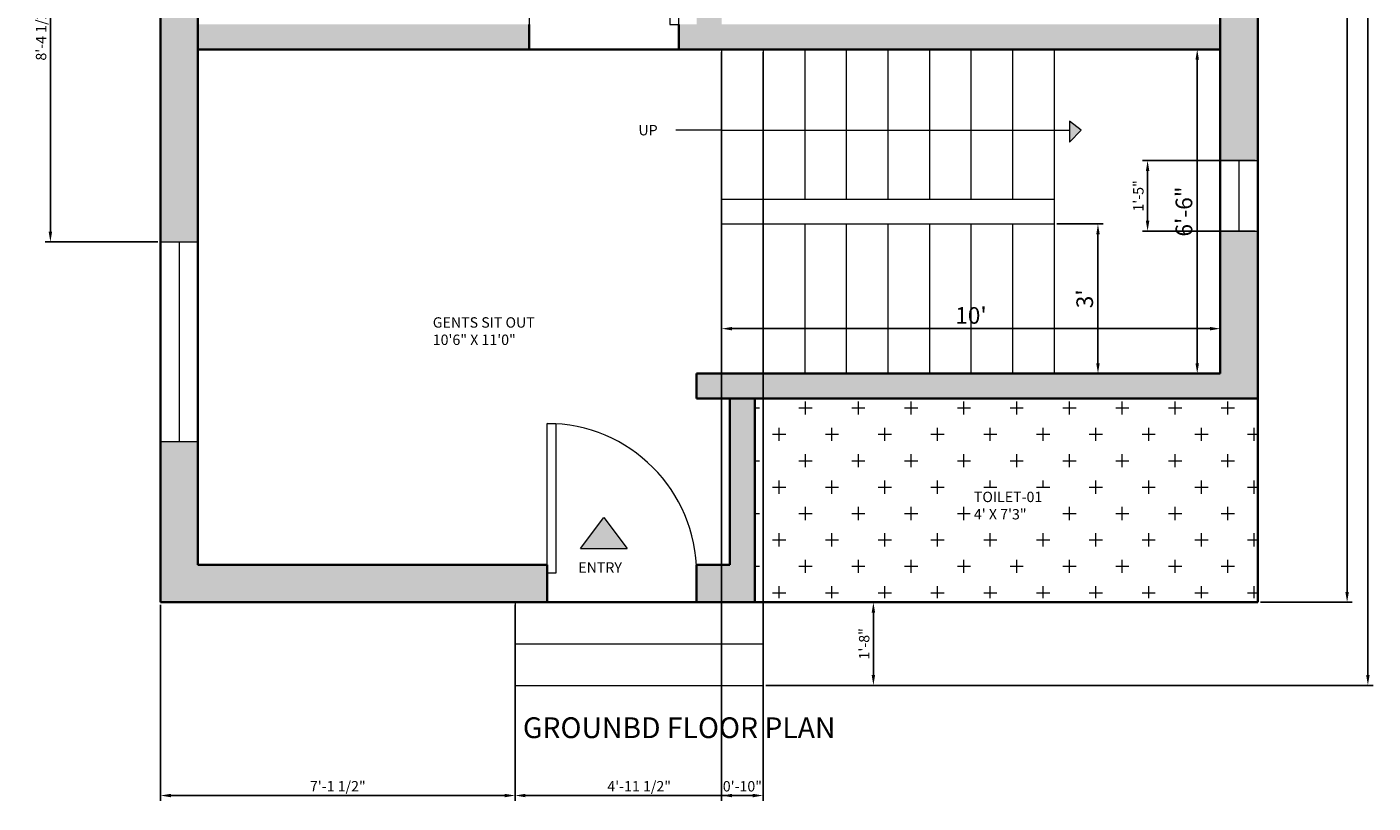
# Model space of a CAD drawing. Units: inches. Extents: x 5395 to 6469, y -203 to 448.
# Tile 6 of 7: x 6145 to 6469, y -203 to -16. Entities that reach past the tile are written whole.
import ezdxf

# ---------------------------------------------------------------- set-up
doc = ezdxf.new("R2010")
doc.units = ezdxf.units.IN
for name, color, linetype, lineweight in [('A-ANNO-DIMS', 2, 'Continuous', 18), ('A-ANNO-SYMB', 3, 'Continuous', 18), ('A-ANNO-TEXT', 6, 'Continuous', 18), ('A-AREA-IDEN', 6, 'Continuous', 18), ('A-FLOR-PATT', 3, 'Continuous', 13), ('A-FLOR-STRS', 3, 'Continuous', 18), ('A-GLAZ', 4, 'Continuous', 18), ('A-WALL', 7, 'Continuous', 35), ('A-WALL-PATT', 11, 'Continuous', 9), ('door', 240, 'Continuous', 18)]:
    doc.layers.add(name, color=color, linetype=linetype, lineweight=lineweight)
doc.styles.get("Standard").update_dxf_attribs({"font": 'arial.ttf'})
doc.dimstyles.new('ISO-25', dxfattribs={"dimtxt": 2.5, "dimasz": 2.5, "dimexe": 1.25, "dimexo": 0.625, "dimtad": 1, "dimdec": 1, "dimlunit": 3, "dimtxsty": 'Standard', "dimcen": 2.5, "dimadec": 0, "dimazin": 0, "dimtfac": 1, "dimtdec": 1, "dimtmove": 0, "dimatfit": 3, "dimfxl": 1, "dimarcsym": 0})

# ---------------------------------------------------------------- blocks, each defined once
blk = doc.blocks.new('*D23')
at = {"layer": 'A-ANNO-DIMS', "color": 0, "lineweight": -2, "transparency": 16777216}
for p, q in [((6421.36, -21.69), (6428.02, -21.69)), ((6426.77, -24.19), (6426.77, -97.19)), ((6427.4, -99.69), (6428.02, -99.69))]:
    blk.add_line(p, q, dxfattribs=at)
at = {"layer": 'A-ANNO-DIMS', "color": 0, "transparency": 16777216}
for points in [[(6426.35, -24.19), (6427.19, -24.19), (6426.77, -21.69)], [(6426.35, -97.19), (6427.19, -97.19), (6426.77, -99.69)]]:
    blk.add_solid(points, dxfattribs=at)
at = {"layer": 'Defpoints', "color": 0, "transparency": 16777216}
for p in [(6420.73, -21.69), (6426.77, -99.69), (6426.77, -99.69)]:
    blk.add_point(p, dxfattribs=at)
at = {"layer": 'A-ANNO-DIMS', "color": 0, "transparency": 16777216, "insert": (6424.1, -60.69), "char_height": 4, "attachment_point": 5, "rotation": 90}
blk.add_mtext('6\'-6"', dxfattribs=at)
blk = doc.blocks.new('*D24')
at = {"layer": 'A-ANNO-DIMS', "color": 0, "lineweight": -2, "transparency": 16777216}
for p, q in [((6392.96, -63.69), (6404.14, -63.69)), ((6402.89, -66.19), (6402.89, -97.19)), ((6392.96, -99.69), (6404.14, -99.69))]:
    blk.add_line(p, q, dxfattribs=at)
at = {"layer": 'A-ANNO-DIMS', "color": 0, "transparency": 16777216}
for points in [[(6402.48, -66.19), (6403.31, -66.19), (6402.89, -63.69)], [(6402.48, -97.19), (6403.31, -97.19), (6402.89, -99.69)]]:
    blk.add_solid(points, dxfattribs=at)
at = {"layer": 'Defpoints', "color": 0, "transparency": 16777216}
for p in [(6392.33, -63.69), (6392.33, -99.69), (6402.89, -99.69)]:
    blk.add_point(p, dxfattribs=at)
at = {"layer": 'A-ANNO-DIMS', "color": 0, "transparency": 16777216, "insert": (6400.22, -81.69), "char_height": 4, "attachment_point": 5, "rotation": 90}
blk.add_mtext("3'", dxfattribs=at)
blk = doc.blocks.new('*D25')
at = {"layer": 'A-ANNO-DIMS', "color": 0, "lineweight": -2, "transparency": 16777216}
for p, q in [((6312.33, -41.76), (6312.33, -90.12)), ((6432.33, -41.76), (6432.33, -90.12)), ((6314.83, -88.87), (6429.83, -88.87))]:
    blk.add_line(p, q, dxfattribs=at)
at = {"layer": 'A-ANNO-DIMS', "color": 0, "transparency": 16777216}
for points in [[(6314.83, -88.46), (6314.83, -89.29), (6312.33, -88.87)], [(6429.83, -88.46), (6429.83, -89.29), (6432.33, -88.87)]]:
    blk.add_solid(points, dxfattribs=at)
at = {"layer": 'Defpoints', "color": 0, "transparency": 16777216}
for p in [(6312.33, -41.13), (6432.33, -41.13), (6432.33, -88.87)]:
    blk.add_point(p, dxfattribs=at)
at = {"layer": 'A-ANNO-DIMS', "color": 0, "transparency": 16777216, "insert": (6372.33, -86.21), "char_height": 4, "attachment_point": 5}
blk.add_mtext("10'", dxfattribs=at)
blk = doc.blocks.new('*U3')
for p, q in [((-30, 0), (-30, -5)), ((0, 0), (0, -5))]:
    blk.add_line(p, q)
blk.add_lwpolyline([(0, 0), (0, 30), (-1.75, 30), (-1.75, 0)], close=True)
blk.add_arc((0, 0), 30, 90, 180)
blk = doc.blocks.new('*U2')
for p, q in [((0, 0), (0, -5)), ((30, 0), (30, -5))]:
    blk.add_line(p, q)
blk.add_lwpolyline([(0, 0), (0, 30), (1.75, 30), (1.75, 0)], close=True)
blk.add_arc((0, 0), 30, 0, 90)
blk = doc.blocks.new('*D28')
at = {"layer": 'A-ANNO-DIMS', "color": 0, "lineweight": -2, "transparency": 16777216}
for p, q in [((6441.96, 325.31), (6464.09, 325.31)), ((6462.84, 322.81), (6462.84, -152.19)), ((6441.96, -154.69), (6464.09, -154.69))]:
    blk.add_line(p, q, dxfattribs=at)
at = {"layer": 'A-ANNO-DIMS', "color": 0, "transparency": 16777216}
for points in [[(6462.42, 322.81), (6463.25, 322.81), (6462.84, 325.31)], [(6462.42, -152.19), (6463.25, -152.19), (6462.84, -154.69)]]:
    blk.add_solid(points, dxfattribs=at)
at = {"layer": 'Defpoints', "color": 0, "transparency": 16777216}
for p in [(6441.33, 325.31), (6441.33, -154.69), (6462.84, -154.69)]:
    blk.add_point(p, dxfattribs=at)
at = {"layer": 'A-ANNO-DIMS', "color": 0, "transparency": 16777216, "insert": (6460.17, 85.31), "char_height": 4, "attachment_point": 5, "rotation": 90}
blk.add_mtext("40'", dxfattribs=at)
blk = doc.blocks.new('WINDOW-48IN')
for p, q in [((0, 0), (0, 9)), ((48, 0), (48, 9)), ((0, 4.5), (48, 4.5))]:
    blk.add_line(p, q)
blk = doc.blocks.new('*D77')
at = {"layer": 'A-ANNO-DIMS', "color": 0, "lineweight": -2, "transparency": 16777216}
for p, q in [((6176.71, 32.67), (6149.58, 32.67)), ((6150.83, 30.17), (6150.83, -65.51)), ((6176.71, -68.01), (6149.58, -68.01))]:
    blk.add_line(p, q, dxfattribs=at)
at = {"layer": 'A-ANNO-DIMS', "color": 0, "transparency": 16777216}
for points in [[(6150.42, 30.17), (6151.25, 30.17), (6150.83, 32.67)], [(6150.42, -65.51), (6151.25, -65.51), (6150.83, -68.01)]]:
    blk.add_solid(points, dxfattribs=at)
at = {"layer": 'Defpoints', "color": 0, "transparency": 16777216}
for p in [(6177.33, 32.67), (6150.83, -68.01), (6177.33, -68.01)]:
    blk.add_point(p, dxfattribs=at)
at = {"layer": 'A-ANNO-DIMS', "color": 0, "transparency": 16777216, "insert": (6148.92, -17.67), "char_height": 2.5, "attachment_point": 5, "rotation": 90}
blk.add_mtext('8\'-4 1/2"', dxfattribs=at)
blk = doc.blocks.new('*D78')
at = {"layer": 'A-ANNO-DIMS', "color": 0, "lineweight": -2, "transparency": 16777216}
for p, q in [((6177.33, -155.32), (6177.33, -202.44)), ((6262.65, -155.32), (6262.65, -202.44)), ((6179.83, -201.19), (6260.15, -201.19))]:
    blk.add_line(p, q, dxfattribs=at)
at = {"layer": 'A-ANNO-DIMS', "color": 0, "transparency": 16777216}
for points in [[(6179.83, -200.78), (6179.83, -201.61), (6177.33, -201.19)], [(6260.15, -200.78), (6260.15, -201.61), (6262.65, -201.19)]]:
    blk.add_solid(points, dxfattribs=at)
at = {"layer": 'Defpoints', "color": 0, "transparency": 16777216}
for p in [(6177.33, -154.69), (6262.65, -154.69), (6262.65, -201.19)]:
    blk.add_point(p, dxfattribs=at)
at = {"layer": 'A-ANNO-DIMS', "color": 0, "transparency": 16777216, "insert": (6219.99, -199.28), "char_height": 2.5, "attachment_point": 5}
blk.add_mtext('7\'-1 1/2"', dxfattribs=at)
blk = doc.blocks.new('*D79')
at = {"layer": 'A-ANNO-DIMS', "color": 0, "lineweight": -2, "transparency": 16777216}
for p, q in [((6262.65, -175.32), (6262.65, -202.44)), ((6322.36, -175.32), (6322.36, -202.44)), ((6265.15, -201.19), (6319.86, -201.19))]:
    blk.add_line(p, q, dxfattribs=at)
at = {"layer": 'A-ANNO-DIMS', "color": 0, "transparency": 16777216}
for points in [[(6265.15, -200.78), (6265.15, -201.61), (6262.65, -201.19)], [(6319.86, -200.78), (6319.86, -201.61), (6322.36, -201.19)]]:
    blk.add_solid(points, dxfattribs=at)
at = {"layer": 'Defpoints', "color": 0, "transparency": 16777216}
for p in [(6262.65, -174.69), (6322.36, -174.69), (6322.36, -201.19)]:
    blk.add_point(p, dxfattribs=at)
at = {"layer": 'A-ANNO-DIMS', "color": 0, "transparency": 16777216, "insert": (6292.5, -199.28), "char_height": 2.5, "attachment_point": 5}
blk.add_mtext('4\'-11 1/2"', dxfattribs=at)
blk = doc.blocks.new('*D80')
at = {"layer": 'A-ANNO-DIMS', "color": 0, "lineweight": -2, "transparency": 16777216}
for p, q in [((6322.98, -154.69), (6350.11, -154.69)), ((6348.86, -157.19), (6348.86, -172.19)), ((6322.98, -174.69), (6350.11, -174.69))]:
    blk.add_line(p, q, dxfattribs=at)
at = {"layer": 'A-ANNO-DIMS', "color": 0, "transparency": 16777216}
for points in [[(6348.44, -157.19), (6349.27, -157.19), (6348.86, -154.69)], [(6348.44, -172.19), (6349.27, -172.19), (6348.86, -174.69)]]:
    blk.add_solid(points, dxfattribs=at)
at = {"layer": 'Defpoints', "color": 0, "transparency": 16777216}
for p in [(6322.36, -154.69), (6322.36, -174.69), (6348.86, -174.69)]:
    blk.add_point(p, dxfattribs=at)
at = {"layer": 'A-ANNO-DIMS', "color": 0, "transparency": 16777216, "insert": (6346.96, -164.69), "char_height": 2.5, "attachment_point": 5, "rotation": 90}
blk.add_mtext('1\'-8"', dxfattribs=at)
blk = doc.blocks.new('*D86')
at = {"layer": 'A-ANNO-DIMS', "color": 0, "lineweight": -2, "transparency": 16777216}
for p, q in [((6440.71, -48.44), (6413.58, -48.44)), ((6414.83, -62.92), (6414.83, -50.94)), ((6440.71, -65.42), (6413.58, -65.42))]:
    blk.add_line(p, q, dxfattribs=at)
at = {"layer": 'A-ANNO-DIMS', "color": 0, "transparency": 16777216}
for points in [[(6414.42, -50.94), (6415.25, -50.94), (6414.83, -48.44)], [(6414.42, -62.92), (6415.25, -62.92), (6414.83, -65.42)]]:
    blk.add_solid(points, dxfattribs=at)
at = {"layer": 'Defpoints', "color": 0, "transparency": 16777216}
for p in [(6414.83, -48.44), (6441.33, -48.44), (6441.33, -65.42)]:
    blk.add_point(p, dxfattribs=at)
at = {"layer": 'A-ANNO-DIMS', "color": 0, "transparency": 16777216, "insert": (6412.93, -56.93), "char_height": 2.5, "attachment_point": 5, "rotation": 90}
blk.add_mtext('1\'-5"', dxfattribs=at)
blk = doc.blocks.new('*D87')
at = {"layer": 'A-ANNO-DIMS', "color": 0, "lineweight": -2, "transparency": 16777216}
for p, q in [((6312.33, -22.32), (6312.33, -202.44)), ((6322.33, -22.32), (6322.33, -202.44)), ((6314.83, -201.19), (6319.83, -201.19))]:
    blk.add_line(p, q, dxfattribs=at)
at = {"layer": 'A-ANNO-DIMS', "color": 0, "transparency": 16777216}
for points in [[(6314.83, -200.78), (6314.83, -201.61), (6312.33, -201.19)], [(6319.83, -200.78), (6319.83, -201.61), (6322.33, -201.19)]]:
    blk.add_solid(points, dxfattribs=at)
at = {"layer": 'Defpoints', "color": 0, "transparency": 16777216}
for p in [(6312.33, -21.69), (6322.33, -21.69), (6322.33, -201.19)]:
    blk.add_point(p, dxfattribs=at)
at = {"layer": 'A-ANNO-DIMS', "color": 0, "transparency": 16777216, "insert": (6317.33, -199.29), "char_height": 2.5, "attachment_point": 5}
blk.add_mtext('0\'-10"', dxfattribs=at)
blk = doc.blocks.new('*D88')
at = {"layer": 'A-ANNO-DIMS', "color": 0, "lineweight": -2, "transparency": 16777216}
for p, q in [((6441.96, 325.31), (6469.08, 325.31)), ((6467.83, -172.19), (6467.83, 322.81)), ((6322.98, -174.69), (6469.08, -174.69))]:
    blk.add_line(p, q, dxfattribs=at)
at = {"layer": 'A-ANNO-DIMS', "color": 0, "transparency": 16777216}
for points in [[(6467.42, 322.81), (6468.25, 322.81), (6467.83, 325.31)], [(6467.42, -172.19), (6468.25, -172.19), (6467.83, -174.69)]]:
    blk.add_solid(points, dxfattribs=at)
at = {"layer": 'Defpoints', "color": 0, "transparency": 16777216}
for p in [(6441.33, 325.31), (6467.83, 325.31), (6322.36, -174.69)]:
    blk.add_point(p, dxfattribs=at)
at = {"layer": 'A-ANNO-DIMS', "color": 0, "transparency": 16777216, "insert": (6465.93, 75.31), "char_height": 2.5, "attachment_point": 5, "rotation": 90}
blk.add_mtext('41\'-8"', dxfattribs=at)

msp = doc.modelspace()

# ---------------------------------------------------------------- hatches: boundary and pattern name
at = {"layer": 'A-ANNO-SYMB'}
h = msp.add_hatch(color=256, dxfattribs=at)
h.dxf.hatch_style = 1
h.paths.add_polyline_path([(6398.86, -41.13), (6396.06, -38.92), (6396.06, -43.98)])
h = msp.add_hatch(color=256, dxfattribs=at)
h.dxf.hatch_style = 1
h.paths.add_polyline_path([(6284.01, -134.32), (6278.42, -141.77), (6289.6, -141.77)])
at = {"layer": 'A-FLOR-PATT'}
h = msp.add_hatch(dxfattribs=at)
h.set_pattern_fill('CROSS', color=256)
h.paths.add_polyline_path([(6441.33, -105.69), (6320.33, -105.69), (6320.33, -153.69), (6441.33, -153.69)])
at = {"layer": 'A-WALL-PATT'}
h = msp.add_hatch(color=256, dxfattribs=at)
h.dxf.hatch_style = 1
h.paths.add_polyline_path([(6278.26, 325.31), (6177.33, 325.31), (6177.33, 299.05), (6186.33, 299.05), (6186.33, 316.31), (6278.26, 316.31)])
h.paths.add_polyline_path([(6186.33, 251.05), (6177.33, 251.05), (6177.33, 160.61), (6186.33, 160.61)])
h.paths.add_polyline_path([(6186.33, 136.61), (6177.33, 136.61), (6177.33, 80.67), (6186.33, 80.67)])
h.paths.add_polyline_path([(6240.33, 152.04), (6234.33, 152.04), (6234.33, 130.31), (6186.33, 130.31), (6186.33, 124.31), (6240.33, 124.31)])
h.paths.add_polyline_path([(6240.33, 196.31), (6186.33, 196.31), (6186.33, 190.31), (6234.33, 190.31), (6234.33, 188.04), (6240.33, 188.04)])
h.paths.add_polyline_path([(6186.33, 32.67), (6177.33, 32.67), (6177.33, -68.01), (6186.33, -68.01)])
h.paths.add_polyline_path([(6266.01, -15.69), (6186.33, -15.69), (6186.33, -21.69), (6266.01, -21.69)])
h.paths.add_polyline_path([(6186.33, -116.01), (6177.33, -116.01), (6177.33, -153.69), (6270.33, -153.69), (6270.33, -145.69), (6186.33, -145.69)])
h.paths.add_polyline_path([(6320.33, -105.69), (6314.33, -105.69), (6314.33, -145.69), (6306.33, -145.69), (6306.33, -153.69), (6320.33, -153.69)])
h.paths.add_polyline_path([(6441.33, -65.42), (6432.33, -65.42), (6432.33, -99.69), (6306.33, -99.69), (6306.33, -105.69), (6441.33, -105.69)])
h.paths.add_polyline_path([(6432.33, -15.69), (6312.33, -15.69), (6312.33, 124.31), (6314.57, 124.31), (6314.57, 130.31), (6306.33, 130.31), (6306.33, -15.69), (6302.01, -15.69), (6302.01, -21.69), (6432.33, -21.69)])
h.paths.add_polyline_path([(6441.33, 25.42), (6432.33, 25.42), (6432.33, -48.44), (6441.33, -48.44)])
h.paths.add_polyline_path([(6441.33, 135.52), (6432.33, 135.52), (6432.33, 130.31), (6432.33, 73.42), (6441.33, 73.42)])
h.paths.add_polyline_path([(6432.33, 130.31), (6350.57, 130.31), (6350.57, 124.31), (6432.33, 124.31)], flags=17)
h.paths.add_polyline_path([(6360.33, 151.9), (6354.33, 151.9), (6354.33, 130.31), (6360.33, 130.31)])
h.paths.add_polyline_path([(6441.33, 251.05), (6432.33, 251.05), (6432.33, 159.52), (6441.33, 159.52)])
h.paths.add_polyline_path([(6432.33, 196.31), (6350.57, 196.31), (6350.57, 190.31), (6354.33, 190.31), (6354.33, 187.9), (6360.33, 187.9), (6360.33, 190.31), (6432.33, 190.31)])
h.paths.add_polyline_path([(6312.33, 316.31), (6306.33, 316.31), (6306.33, 196.31), (6297.04, 196.31), (6297.04, 190.31), (6306.33, 190.31), (6314.57, 190.31), (6314.57, 196.31), (6312.33, 196.31)])
h.paths.add_polyline_path([(6441.33, 325.31), (6302.26, 325.31), (6302.26, 316.31), (6432.33, 316.31), (6432.33, 299.05), (6441.33, 299.05)])
h = msp.add_hatch(color=256, dxfattribs=at)
h.dxf.hatch_style = 1
h.paths.add_polyline_path([(6320.33, -153.69), (6320.33, -105.69), (6314.33, -105.69), (6314.33, -145.69), (6306.33, -145.69), (6306.33, -153.69), (6306.33, -154.69), (6320.33, -154.69)])
h = msp.add_hatch(color=256, dxfattribs=at)
h.dxf.hatch_style = 1
h.paths.add_polyline_path([(6270.33, -153.69), (6270.33, -145.69), (6186.33, -145.69), (6186.33, -116.01), (6177.33, -116.01), (6177.33, -153.69), (6177.33, -154.69), (6270.33, -154.69)])

# ---------------------------------------------------------------- linework, layer by layer
at = {"layer": 'A-ANNO-SYMB'}
for p, q in [((6312.33, -41.13), (6301.33, -41.13)), ((6312.33, -41.13), (6396.06, -41.13)), ((6398.86, -41.13), (6396.06, -38.92)), ((6396.06, -38.92), (6396.06, -43.98)), ((6396.06, -43.98), (6398.86, -41.13)), ((6278.42, -141.77), (6284.01, -134.32)), ((6284.01, -134.32), (6289.6, -141.77)), ((6278.42, -141.77), (6289.6, -141.77))]:
    msp.add_line(p, q, dxfattribs=at)
at = {"layer": 'A-FLOR-STRS'}
for p, q in [((6312.33, -57.69), (6392.33, -57.69)), ((6312.33, -63.69), (6392.33, -63.69)), ((6262.65, -154.69), (6262.65, -174.69)), ((6322.36, -174.69), (6322.36, -154.69)), ((6262.65, -164.69), (6322.36, -164.69)), ((6262.65, -174.69), (6322.36, -174.69))]:
    msp.add_line(p, q, dxfattribs=at)
for points in [[(6312.33, -21.69), (6312.33, -99.69)], [(6312.33, -21.69), (6312.33, -99.69)], [(6322.33, -21.69), (6322.33, -57.69)], [(6332.33, -21.69), (6332.33, -57.69)], [(6342.33, -21.69), (6342.33, -57.69)], [(6352.33, -21.69), (6352.33, -57.69)], [(6362.33, -21.69), (6362.33, -57.69)], [(6372.33, -21.69), (6372.33, -57.69)], [(6382.33, -21.69), (6382.33, -57.69)], [(6392.33, -21.69), (6392.33, -99.69)], [(6322.33, -63.69), (6322.33, -99.69)], [(6332.33, -63.69), (6332.33, -99.69)], [(6342.33, -63.69), (6342.33, -99.69)], [(6352.33, -63.69), (6352.33, -99.69)], [(6362.33, -63.69), (6362.33, -99.69)], [(6372.33, -63.69), (6372.33, -99.69)], [(6382.33, -63.69), (6382.33, -99.69)]]:
    msp.add_lwpolyline(points, dxfattribs=at)
at = {"layer": 'A-GLAZ'}
for p, q in [((6432.33, -48.44), (6441.33, -48.44)), ((6436.83, -65.42), (6436.83, -48.44)), ((6432.33, -65.42), (6441.33, -65.42))]:
    msp.add_line(p, q, dxfattribs=at)
at = {"layer": 'A-WALL'}
for p, q in [((6177.33, -153.69), (6177.33, 325.31)), ((6441.33, -153.69), (6441.33, 325.31)), ((6186.33, -145.69), (6186.33, 316.31)), ((6432.33, -99.69), (6432.33, 316.31)), ((6266.01, -15.69), (6266.01, -21.69)), ((6302.01, -15.69), (6302.01, -21.69)), ((6186.33, -21.69), (6432.33, -21.69)), ((6306.33, -99.69), (6432.33, -99.69)), ((6306.33, -99.69), (6306.33, -105.69)), ((6306.33, -105.69), (6441.33, -105.69)), ((6186.33, -145.69), (6270.33, -145.69)), ((6270.33, -145.69), (6270.33, -153.69)), ((6306.33, -145.69), (6306.33, -153.69)), ((6306.33, -145.69), (6314.33, -145.69)), ((6177.33, -153.69), (6177.33, -154.69)), ((6177.33, -154.69), (6441.33, -154.69)), ((6270.33, -153.69), (6270.33, -154.69)), ((6306.33, -153.69), (6306.33, -154.69)), ((6320.33, -153.69), (6320.33, -154.69))]:
    msp.add_line(p, q, dxfattribs=at)
for points in [[(6432.33, -21.69), (6432.33, -99.69)], [(6314.33, -105.69), (6314.33, -145.69)], [(6320.33, -105.69), (6320.33, -153.69)], [(6441.33, -105.69), (6441.33, -154.69)]]:
    msp.add_lwpolyline(points, dxfattribs=at)

# ---------------------------------------------------------------- block references
at = {"layer": 'A-GLAZ', "rotation": 269.999999999997}
msp.add_blockref('WINDOW-48IN', (6177.33, -68.01), dxfattribs=at)
at = {"layer": 'door', "xscale": 1.199999999999999, "yscale": 1.199999999999999, "zscale": 1.199999999999999}
for name, p in [('*U3', (6302.01, -15.69)), ('*U2', (6270.33, -147.69))]:
    msp.add_blockref(name, p, dxfattribs=at)

# ---------------------------------------------------------------- texts
at = {"layer": 'A-ANNO-TEXT', "attachment_point": 1}
for s, width, insert, char_height in [('              UP', 62.1492, (6281.63, -39.87), 2.5), ('    ENTRY', 62.1492, (6274.8, -145.09), 2.5), ('GROUNBD FLOOR PLAN', 95.1044, (6264.53, -182.38), 5)]:
    msp.add_mtext_dynamic_manual_height_columns(s, width=width, gutter_width=12.5, heights=[0], dxfattribs=dict(at, insert=insert, char_height=char_height))
at = {"layer": 'A-AREA-IDEN', "insert": (6242.84, -86.13), "char_height": 2.5, "attachment_point": 1}
msp.add_mtext_dynamic_manual_height_columns('GENTS SIT OUT\\P10\'6" X 11\'0"', width=62.1492, gutter_width=12.5, heights=[0], dxfattribs=at)

# ---------------------------------------------------------------- dimensions: what is measured, and where the dimension line sits
at = {"layer": 'A-ANNO-DIMS'}
for base, p1, p2, angle, override, picture, middle in [((6462.84, -154.69), (6441.33, 325.31), (6441.33, -154.69), 90, {"dimtxt": 4, "dimclrd": 0, "dimclre": 0, "dimclrt": 0}, '*D28', (6460.17, 85.31)), ((6150.83, -68.01), (6177.33, 32.67), (6177.33, -68.01), 90, {"dimdec": 1, "dimlfac": 1, "dimrnd": 0, "dimzin": 1, "dimdsep": 46, "dimlunit": 4, "dimfrac": 2}, '*D77', (6148.92, -17.67)), ((6426.77, -99.69), (6420.73, -21.69), (6426.77, -99.69), 90, {"dimtxt": 4, "dimclrd": 0, "dimclre": 0, "dimclrt": 0}, '*D23', (6424.1, -60.69)), ((6414.83, -48.44), (6441.33, -65.42), (6441.33, -48.44), 90, {"dimdec": 1, "dimlfac": 1, "dimrnd": 0, "dimzin": 1, "dimdsep": 46, "dimlunit": 4, "dimfrac": 2}, '*D86', (6412.93, -56.93)), ((6402.89, -99.69), (6392.33, -63.69), (6392.33, -99.69), 90, {"dimtxt": 4, "dimclrd": 0, "dimclre": 0, "dimclrt": 0}, '*D24', (6400.22, -81.69)), ((6348.86, -174.69), (6322.36, -154.69), (6322.36, -174.69), 270, {"dimdec": 1, "dimlfac": 1, "dimrnd": 0, "dimzin": 1, "dimdsep": 46, "dimlunit": 4, "dimfrac": 2}, '*D80', (6346.96, -164.69))]:
    dim = msp.add_linear_dim(base=base, p1=p1, p2=p2, angle=angle, dimstyle='ISO-25', override=override, dxfattribs=at)
    dim.commit()
    dim.dimension.update_dxf_attribs({"geometry": picture, "text_midpoint": middle})
for base, p1, p2, override, picture, middle in [((6322.33, -201.19), (6312.33, -21.69), (6322.33, -21.69), {"dimdec": 1, "dimlfac": 1, "dimrnd": 0, "dimzin": 1, "dimdsep": 46, "dimlunit": 4, "dimfrac": 2}, '*D87', (6317.33, -199.29)), ((6432.33, -88.87), (6312.33, -41.13), (6432.33, -41.13), {"dimtxt": 4, "dimclrd": 0, "dimclre": 0, "dimclrt": 0}, '*D25', (6372.33, -86.21)), ((6262.65, -201.19), (6177.33, -154.69), (6262.65, -154.69), {"dimdec": 1, "dimlfac": 1, "dimrnd": 0, "dimzin": 1, "dimdsep": 46, "dimlunit": 4, "dimfrac": 2}, '*D78', (6219.99, -199.28)), ((6322.36, -201.19), (6262.65, -174.69), (6322.36, -174.69), {"dimdec": 1, "dimlfac": 1, "dimrnd": 0, "dimzin": 1, "dimdsep": 46, "dimlunit": 4, "dimfrac": 2}, '*D79', (6292.5, -199.28))]:
    dim = msp.add_linear_dim(base=base, p1=p1, p2=p2, dimstyle='ISO-25', override=override, dxfattribs=at)
    dim.commit()
    dim.dimension.update_dxf_attribs({"geometry": picture, "text_midpoint": middle})

# ---------------------------------------------------------------- next in the draw order: wipeouts: each hides what was drawn before it
msp.add_wipeout([(6372.16, -135.74), (6390.46, -135.74), (6390.46, -127.22), (6372.16, -127.22)]).dxf.layer = 'A-AREA-IDEN'

# ---------------------------------------------------------------- next in the draw order: texts
at = {"layer": 'A-AREA-IDEN', "insert": (6373.04, -128.1), "char_height": 2.5, "width": 62.1492, "attachment_point": 1}
msp.add_mtext('TOILET-01\\P4\' X 7\'3"', dxfattribs=at)

# ---------------------------------------------------------------- next in the draw order: dimensions: what is measured, and where the dimension line sits
at = {"layer": 'A-ANNO-DIMS'}
dim = msp.add_linear_dim(base=(6467.83, 325.31), p1=(6322.36, -174.69), p2=(6441.33, 325.31), angle=90, dimstyle='ISO-25', override={"dimdec": 1, "dimlfac": 1, "dimrnd": 0, "dimzin": 1, "dimdsep": 46, "dimlunit": 4, "dimfrac": 2}, dxfattribs=at)
dim.commit()
dim.dimension.update_dxf_attribs({"geometry": '*D88', "text_midpoint": (6465.93, 75.31)})

doc.saveas('drawing.dxf')
